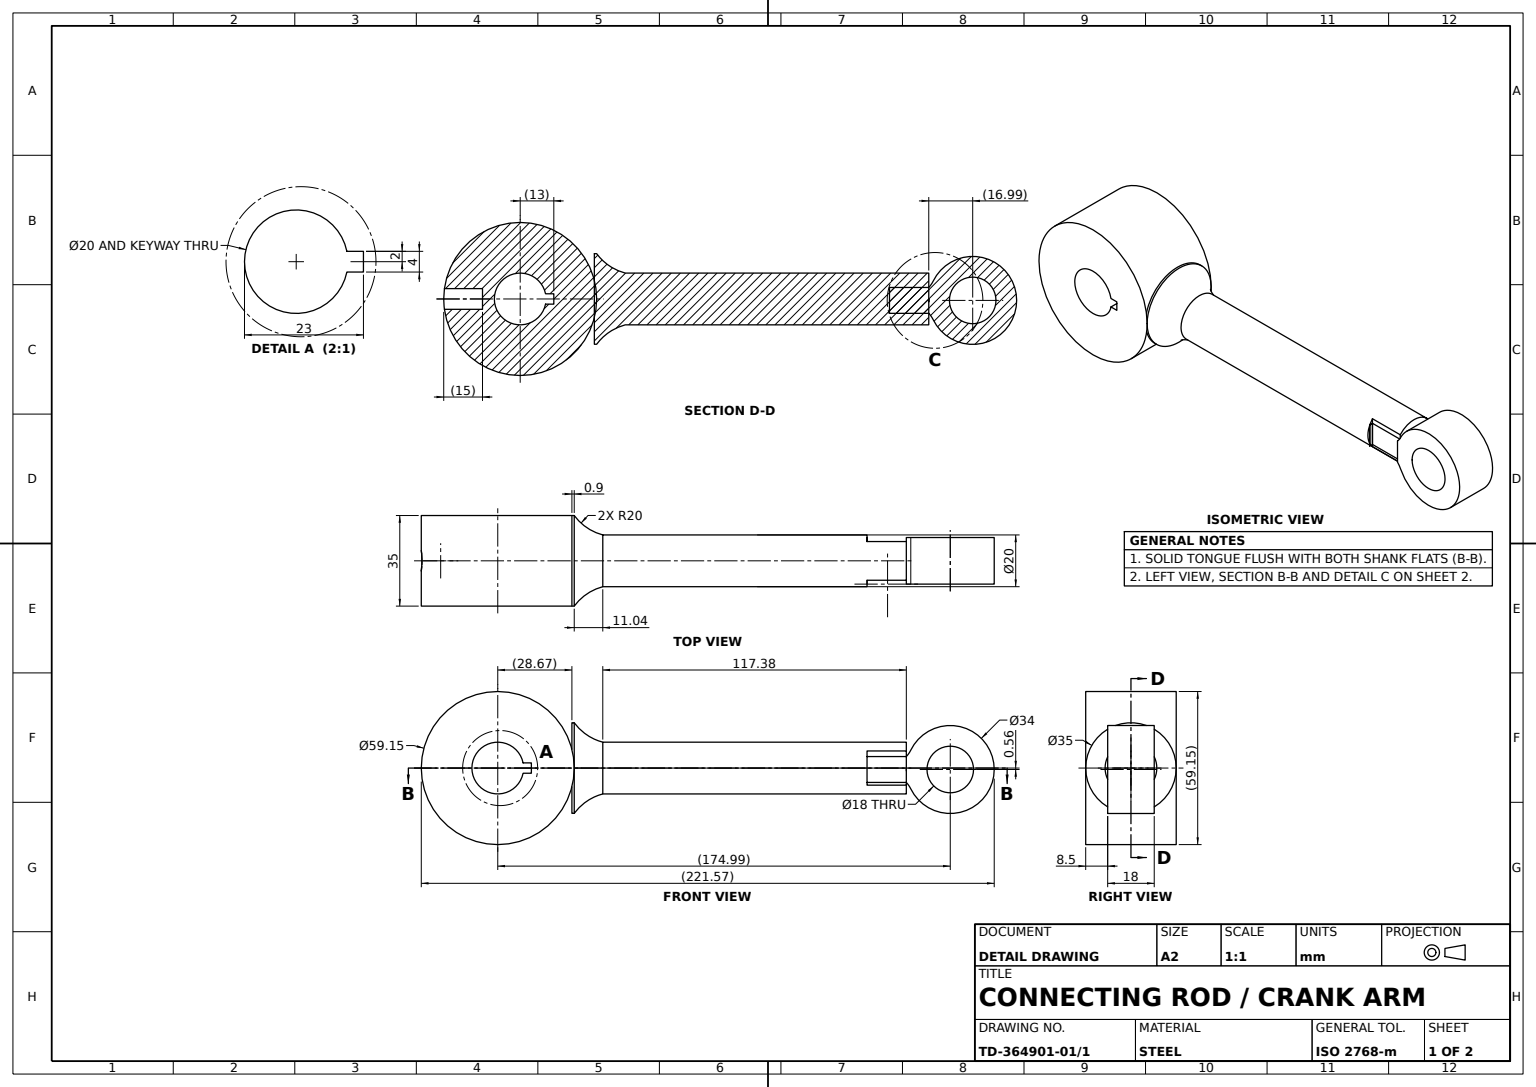
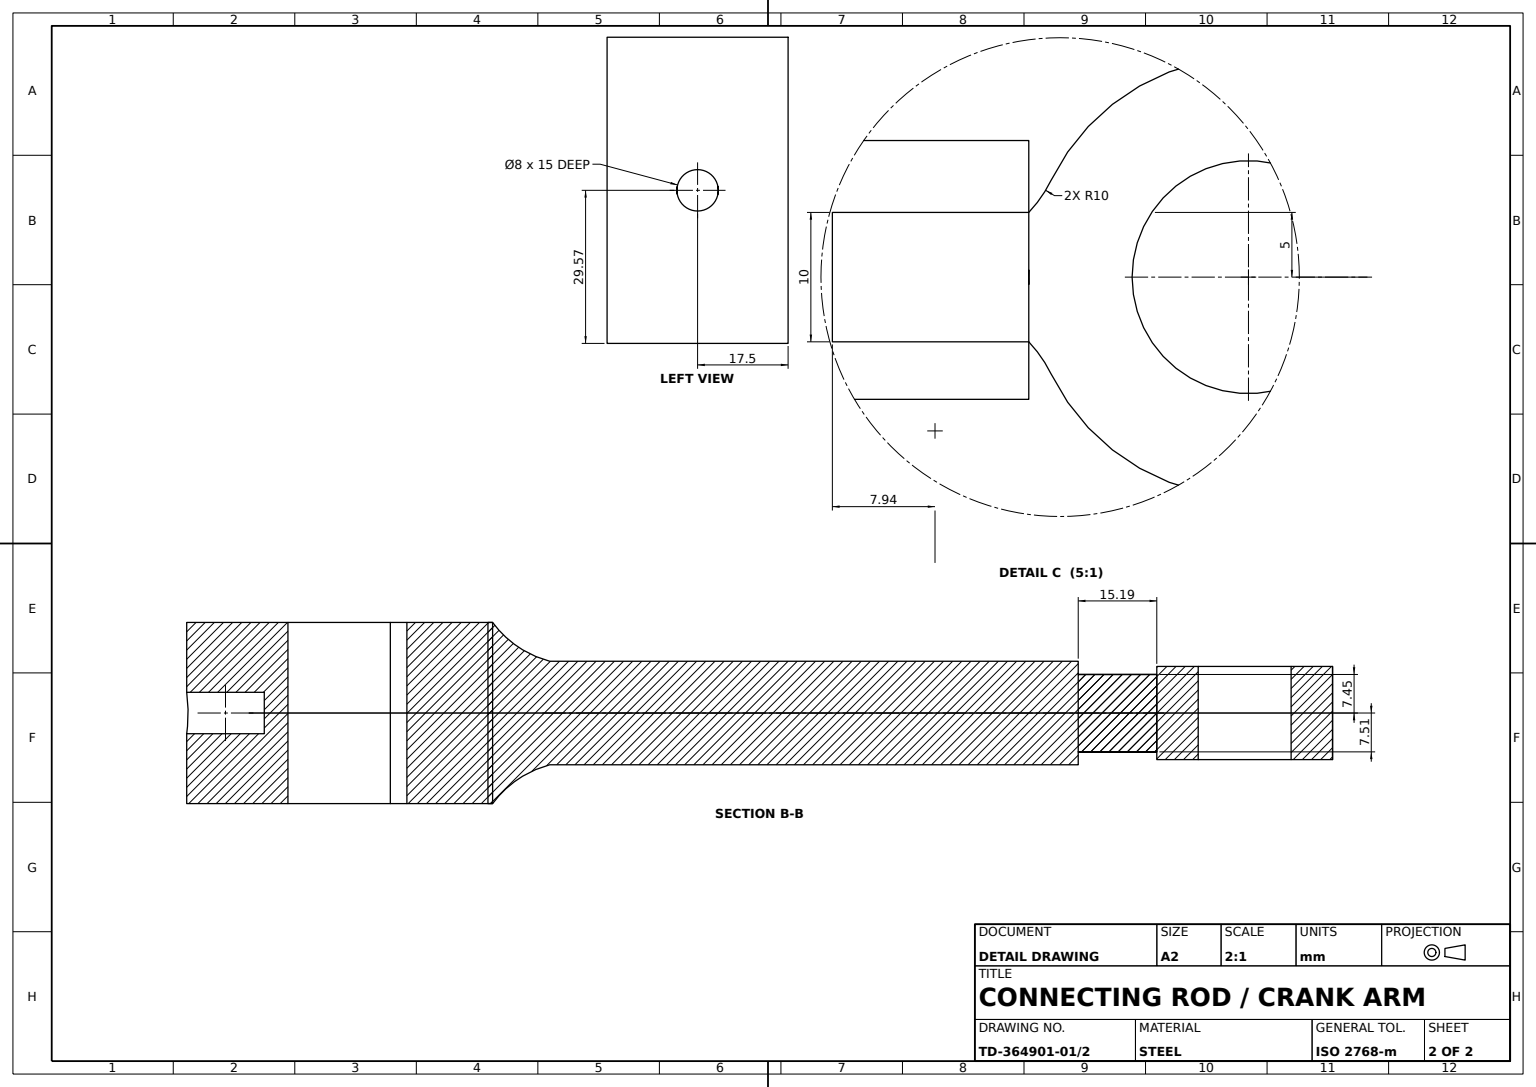
from build123d import *

# Parameters (mm, degrees)
ROD_SHANK_PROFILE_W           = 117.383003688
ROD_SHANK_PROFILE_H           = 10
BIG_END_EYE_PROFILE_R         = 29.574575968
BIG_END_EYE_DEPTH             = 17.5
SMALL_END_EYE_DEPTH           = 9
SMALL_END_FLAT_CUT_DEPTH      = 190.138912872
SMALL_END_FLAT_CUT_DEPTH_BACK = 190.138912872
SMALL_END_FLAT_PROFILE_W      = 15.191641878
SMALL_END_FLAT_PROFILE_H      = 5.882566039
SMALL_END_FLAT_PROFILE_H_2    = 8.578742141
BIG_END_HUB_PROFILE_W         = 15
BIG_END_HUB_PROFILE_H         = 4
BIG_END_KEYWAY_PROFILE_R      = 4
BIG_END_KEYWAY_CUT_DEPTH      = 15


with BuildPart() as part:
    # Rod Shank Profile → Rod Shank (revolve)
    with BuildSketch(Plane.XY, mode=Mode.PRIVATE) as rod_shank_sk:
        with Locations((93.308498156, 5)):
            Rectangle(ROD_SHANK_PROFILE_W, ROD_SHANK_PROFILE_H)
    revolve(rod_shank_sk.sketch.rotate(Axis((0, 0, 0), (1, 0, 0)), 90), axis=Axis((0, 0, 0), (1, 0, 0)))

    # Big End Neck Profile → Big End Neck (revolve)
    with BuildSketch(Plane(origin=(0, 0, 0), x_dir=(1, 0, 0), z_dir=(0, 1, 0))):
        with BuildLine():
            Line((34.616996312, 10), (34.616996312, 0))
            Line((34.616996312, 0), (23.574575968, 0))
            Line((23.574575968, 0), (22.673236665, 0))
            Line((22.673236665, 0), (22.673236665, 17.5))
            Line((22.673236665, 17.5), (23.574575968, 17.5))
            ThreePointArc((23.574575968, 17.5), (28.451606539, 12.801559743), (34.616996312, 10))
        make_face()
    revolve(axis=Axis((34.616996312, 0, 0), (-1, 0, 0)))


with BuildPart() as body_2:
    # Big End Eye Profile → Big End Eye (new, symmetric)
    with BuildSketch(Plane.XY):
        with Locations((-6, 0)):
            Circle(BIG_END_EYE_PROFILE_R)
        with BuildLine():
            ThreePointArc((3.797958971, 2), (-16, 0), (3.797958971, -2))
            Line((3.797958971, -2), (7, -2))
            Line((7, -2), (7, 2))
            Line((7, 2), (3.797958971, 2))
        make_face(mode=Mode.SUBTRACT)
    extrude(amount=BIG_END_EYE_DEPTH, both=True)

    # Big End Hub Profile → Big End Hub (revolve)
    with BuildSketch(Plane(origin=(0, 0, 0), x_dir=(1, 0, 0), z_dir=(0, 1, 0))):
        with Locations((-28.074575968, 2)):
            Rectangle(BIG_END_HUB_PROFILE_W, BIG_END_HUB_PROFILE_H)
    revolve(axis=Axis((-35.574575968, 0, 0), (1, 0, 0)))

    # Big End Keyway Profile → Big End Keyway Cut (cut)
    with BuildSketch(Plane.ZY.offset(35.574575968)):
        Circle(BIG_END_KEYWAY_PROFILE_R)
    extrude(amount=-BIG_END_KEYWAY_CUT_DEPTH, mode=Mode.SUBTRACT)


with BuildPart() as body_3:
    # Small End Eye Profile → Small End Eye (new, symmetric)
    # profile 1 of 2: a face of its own
    with BuildSketch(Plane.XY):
        with BuildLine():
            Line((152, -1.111021517), (152, -5.555510758))
            ThreePointArc((152, -5.555510758), (152.957579332, -6.731309244), (153.726364566, -8.038378301))
            ThreePointArc((153.726364566, -8.038378301), (185.990921335, -0.555510758), (153.726364566, 6.927356785))
            ThreePointArc((153.726364566, 6.927356785), (152.957579332, 5.620287727), (152, 4.444489242))
            Line((152, 4.444489242), (152, 0))
            Line((152, 0), (152, -1.111021517))
        make_face()
        with BuildLine():
            ThreePointArc((161.507606561, -5.555510758), (166.378435254, 8.056975322), (177.990921335, -0.555510758))
            ThreePointArc((177.990921335, -0.555510758), (171.603407415, -9.167996839), (161.507606561, -5.555510758))
        make_face(mode=Mode.SUBTRACT)
    # profile 2 of 2: a face of its own
    with BuildSketch(Plane.XY):
        with BuildLine():
            Line((136.808163002, -5.555510758), (152, -5.555510758))
            Line((152, -5.555510758), (152, -1.111021517))
            ThreePointArc((152, -1.111021517), (151.990921335, -0.555510758), (152, 0))
            Line((152, 0), (152, 4.444489242))
            Line((152, 4.444489242), (136.808163002, 4.444489242))
            Line((136.808163002, 4.444489242), (136.808163002, -5.555510758))
        make_face()
    extrude(amount=SMALL_END_EYE_DEPTH, both=True)


with BuildPart() as small_end_flat_cut_tool:
    # Small End Flat Profile → Small End Flat Cut (new, two sides: drawn at the far end of the back side and taken through both)
    with BuildSketch(Plane(origin=(0, 0, 0), x_dir=(1, 0, 0), z_dir=(0, 1, 0)).offset(-SMALL_END_FLAT_CUT_DEPTH_BACK)):
        with Locations((144.404179061, -10.446972753)):
            Rectangle(SMALL_END_FLAT_PROFILE_W, SMALL_END_FLAT_PROFILE_H)
        with Locations((144.404179061, 11.735203356)):
            Rectangle(SMALL_END_FLAT_PROFILE_W, SMALL_END_FLAT_PROFILE_H_2)
    extrude(amount=SMALL_END_FLAT_CUT_DEPTH + SMALL_END_FLAT_CUT_DEPTH_BACK)


with BuildPart() as part_1:
    add(part.part)

    # Small End Flat Cut: cut by small_end_flat_cut_tool
    add(small_end_flat_cut_tool.part, mode=Mode.SUBTRACT)


with BuildPart() as body_3_1:
    add(body_3.part)

    # Small End Flat Cut: cut by small_end_flat_cut_tool
    add(small_end_flat_cut_tool.part, mode=Mode.SUBTRACT)


solid = Compound([body_2.part, part_1.part, body_3_1.part])
